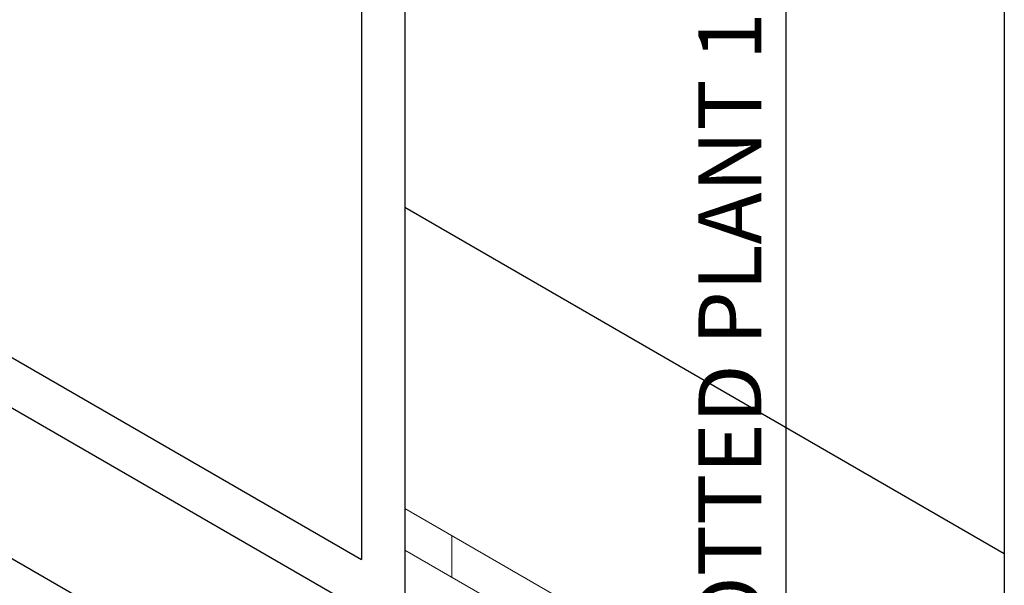
# Model space of a CAD drawing. Units: inches. Extents: x 5770 to 11891, y 3254 to 6808.
# Tile 11 of 15: x 6034 to 6073, y 3436 to 3459. Entities that reach past the tile are written whole.
import ezdxf

# ---------------------------------------------------------------- set-up
doc = ezdxf.new("R2010")
doc.units = ezdxf.units.IN
for name, color, linetype, lineweight in [('A-ANNO-DIMS', 2, 'Continuous', 18), ('A-DOOR', 4, 'Continuous', 25), ('A-FURN', 8, 'Continuous', 25), ('A-GLAZ', 4, 'Continuous', 25), ('A-WALL-PATT', 8, 'Continuous', 13)]:
    doc.layers.add(name, color=color, linetype=linetype, lineweight=lineweight)
doc.styles.get("Standard").update_dxf_attribs({"font": 'arial.ttf'})
doc.dimstyles.new('ISO-25', dxfattribs={"dimtxt": 2.5, "dimasz": 2.5, "dimexe": 1.25, "dimexo": 0.625, "dimtad": 1, "dimdec": 0, "dimlunit": 3, "dimtxsty": 'Standard', "dimcen": 2.5, "dimadec": 0, "dimazin": 0, "dimtfac": 1, "dimtdec": 0, "dimtmove": 0, "dimatfit": 3, "dimfxl": 1, "dimarcsym": 0})

# ---------------------------------------------------------------- blocks, each defined once
blk = doc.blocks.new('*D7')
at = {"layer": 'A-ANNO-DIMS', "color": 0, "lineweight": -2, "transparency": 16777216}
for p, q in [((5959.627, 3549.37), (5966.461, 3561.208)), ((5968.001, 3558.875), (6136.876, 3461.375)), ((6132.832, 3449.37), (6139.666, 3461.208))]:
    blk.add_line(p, q, dxfattribs=at)
at = {"layer": 'A-ANNO-DIMS', "color": 0, "transparency": 16777216}
for points in [[(5968.21, 3559.236), (5967.793, 3558.514), (5965.836, 3560.125)], [(6137.085, 3461.736), (6136.668, 3461.014), (6139.041, 3460.125)]]:
    blk.add_solid(points, dxfattribs=at)
at = {"layer": 'Defpoints', "color": 0, "transparency": 16777216}
for p in [(5959.314, 3548.829), (6139.041, 3460.125), (6132.519, 3448.829)]:
    blk.add_point(p, dxfattribs=at)
at = {"layer": 'A-ANNO-DIMS', "color": 0, "transparency": 16777216, "insert": (6061.618, 3507.021), "char_height": 2.5, "attachment_point": 5, "rotation": 330}
blk.add_mtext('16\'-8"', dxfattribs=at)
blk = doc.blocks.new('*D38')
at = {"layer": 'A-ANNO-DIMS', "color": 0, "lineweight": -2, "transparency": 16777216}
for p, q in [((6064.558, 3428.516), (6064.558, 3471.974)), ((6062.594, 3428.516), (6065.808, 3428.516)), ((6064.558, 3413.754), (6064.558, 3426.016)), ((6062.594, 3411.254), (6065.808, 3411.254))]:
    blk.add_line(p, q, dxfattribs=at)
at = {"layer": 'A-ANNO-DIMS', "color": 0, "transparency": 16777216}
for points in [[(6064.141, 3426.016), (6064.975, 3426.016), (6064.558, 3428.516)], [(6064.141, 3413.754), (6064.975, 3413.754), (6064.558, 3411.254)]]:
    blk.add_solid(points, dxfattribs=at)
at = {"layer": 'Defpoints', "color": 0, "transparency": 16777216}
for p in [(6061.969, 3428.516), (6064.558, 3428.516), (6061.969, 3411.254)]:
    blk.add_point(p, dxfattribs=at)
at = {"layer": 'A-ANNO-DIMS', "color": 0, "transparency": 16777216, "insert": (6062.64, 3451.495), "char_height": 2.5, "attachment_point": 5, "rotation": 90}
blk.add_mtext('POTTED PLANT 1\'-5 1/2"', dxfattribs=at)

msp = doc.modelspace()

# ---------------------------------------------------------------- linework, layer by layer
at = {"layer": 'A-DOOR'}
msp.add_line((6073.257, 3462.723), (6073.257, 3386.42), dxfattribs=at)
at = {"layer": 'A-FURN'}
for p, q in [((6049.365, 3476.517), (6049.365, 3434.517)), ((6049.365, 3451.555), (6073.257, 3437.761)), ((6016.362, 3447.572), (6044.169, 3431.517))]:
    msp.add_line(p, q, dxfattribs=at)
at = {"layer": 'A-GLAZ'}
for p, q in [((6047.633, 3475.517), (6047.633, 3437.517)), ((6009.528, 3459.517), (6047.633, 3437.517)), ((6007.795, 3458.517), (6049.365, 3434.517))]:
    msp.add_line(p, q, dxfattribs=at)
at = {"layer": 'A-WALL-PATT'}
for p, q in [((6049.365, 3439.555), (6073.257, 3425.761)), ((6051.234, 3438.476), (6051.234, 3436.815)), ((6049.365, 3437.894), (6073.257, 3424.1))]:
    msp.add_line(p, q, dxfattribs=at)

# ---------------------------------------------------------------- dimensions: what is measured, and where the dimension line sits
at = {"layer": 'A-ANNO-DIMS'}
dim = msp.add_linear_dim(base=(6139.041, 3460.125), p1=(5959.314, 3548.829), p2=(6132.519, 3448.829), angle=330, dimstyle='ISO-25', override={"dimclrd": 0, "dimclre": 0, "dimclrt": 0}, dxfattribs=at)
dim.commit()
dim.dimension.update_dxf_attribs({"geometry": '*D7', "text_midpoint": (6060.667, 3505.374), "dimtype": 161})
dim = msp.add_linear_dim(base=(6064.558, 3428.516), p1=(6061.969, 3411.254), p2=(6061.969, 3428.516), angle=90, text='POTTED PLANT <>', dimstyle='ISO-25', override={"dimdec": 1, "dimlfac": 1, "dimrnd": 0, "dimzin": 1, "dimdsep": 46, "dimlunit": 4, "dimfrac": 2}, dxfattribs=at)
dim.commit()
dim.dimension.update_dxf_attribs({"geometry": '*D38', "text_midpoint": (6062.64, 3451.495)})

doc.saveas('drawing.dxf')
